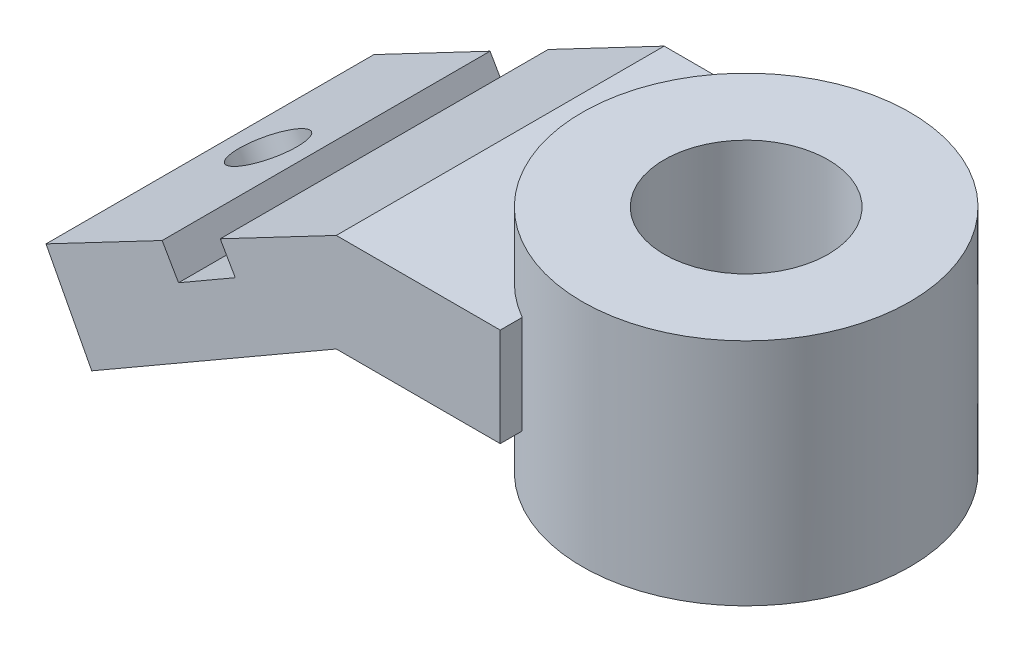
ISO-10303-21;
HEADER;
FILE_DESCRIPTION(('STEP AP214'),'2;1');
FILE_NAME('part.step','',(''),(''),'','','');
FILE_SCHEMA(('AUTOMOTIVE_DESIGN { 1 0 10303 214 1 1 1 1 }'));
ENDSEC;
DATA;
#1=APPLICATION_CONTEXT('core data for automotive mechanical design processes');
#2=APPLICATION_PROTOCOL_DEFINITION('international standard','automotive_design',2000,#1);
#3=PRODUCT_CONTEXT('',#1,'mechanical');
#4=PRODUCT('Part','Part','',(#3));
#5=PRODUCT_RELATED_PRODUCT_CATEGORY('part','',(#4));
#6=PRODUCT_DEFINITION_FORMATION('','',#4);
#7=PRODUCT_DEFINITION_CONTEXT('part definition',#1,'design');
#8=PRODUCT_DEFINITION('design','',#6,#7);
#9=PRODUCT_DEFINITION_SHAPE('','',#8);
#10=(LENGTH_UNIT() NAMED_UNIT(*) SI_UNIT(.MILLI.,.METRE.));
#11=(NAMED_UNIT(*) PLANE_ANGLE_UNIT() SI_UNIT($,.RADIAN.));
#12=(NAMED_UNIT(*) SI_UNIT($,.STERADIAN.) SOLID_ANGLE_UNIT());
#13=UNCERTAINTY_MEASURE_WITH_UNIT(LENGTH_MEASURE(1.E-05),#10,'distance_accuracy_value','');
#14=(GEOMETRIC_REPRESENTATION_CONTEXT(3) GLOBAL_UNCERTAINTY_ASSIGNED_CONTEXT((#13)) GLOBAL_UNIT_ASSIGNED_CONTEXT((#10,
#11,#12)) REPRESENTATION_CONTEXT('',''));
#15=CARTESIAN_POINT('',(0.,0.,0.));
#16=DIRECTION('',(0.,0.,1.));
#17=DIRECTION('',(1.,0.,0.));
#18=AXIS2_PLACEMENT_3D('',#15,#16,#17);
#19=CARTESIAN_POINT('',(-69.2655182091907,-8.25003005743869,25.));
#20=DIRECTION('',(0.465000601148774,-0.885310364183815,0.));
#21=DIRECTION('',(0.885310364183815,0.465000601148774,0.));
#22=AXIS2_PLACEMENT_3D('',#19,#20,#21);
#23=PLANE('',#22);
#24=DIRECTION('',(0.,0.,1.));
#25=VECTOR('',#24,1.);
#26=CARTESIAN_POINT('',(-42.7026701508798,5.70184582139558,-25.));
#27=LINE('',#26,#25);
#28=CARTESIAN_POINT('',(-42.7026701508798,5.70184582139558,-25.));
#29=VERTEX_POINT('',#28);
#30=CARTESIAN_POINT('',(-42.7026701508798,5.70184582139558,25.));
#31=VERTEX_POINT('',#30);
#32=EDGE_CURVE('E167',#29,#31,#27,.T.);
#33=ORIENTED_EDGE('',*,*,#32,.T.);
#34=DIRECTION('',(-0.885310364183815,-0.465000601148774,0.));
#35=VECTOR('',#34,1.);
#36=CARTESIAN_POINT('',(-69.2655182091907,-8.25003005743869,25.));
#37=LINE('',#36,#35);
#38=CARTESIAN_POINT('',(-25.,15.,25.));
#39=VERTEX_POINT('',#38);
#40=EDGE_CURVE('E196',#39,#31,#37,.T.);
#41=ORIENTED_EDGE('',*,*,#40,.F.);
#42=DIRECTION('',(0.,0.,-1.));
#43=VECTOR('',#42,1.);
#44=CARTESIAN_POINT('',(-25.,15.,25.));
#45=LINE('',#44,#43);
#46=CARTESIAN_POINT('',(-25.,15.,-25.));
#47=VERTEX_POINT('',#46);
#48=EDGE_CURVE('E233',#39,#47,#45,.T.);
#49=ORIENTED_EDGE('',*,*,#48,.T.);
#50=DIRECTION('',(-0.885310364183815,-0.465000601148774,0.));
#51=VECTOR('',#50,1.);
#52=CARTESIAN_POINT('',(-69.2655182091907,-8.25003005743869,-25.));
#53=LINE('',#52,#51);
#54=EDGE_CURVE('E215',#47,#29,#53,.T.);
#55=ORIENTED_EDGE('',*,*,#54,.T.);
#56=EDGE_LOOP('',(#33,#41,#49,#55));
#57=FACE_BOUND('',#56,.T.);
#58=ADVANCED_FACE('F43',(#57),#23,.F.);
#59=CARTESIAN_POINT('',(0.,0.,25.));
#60=DIRECTION('',(-1.,0.,0.));
#61=DIRECTION('',(0.,0.,1.));
#62=AXIS2_PLACEMENT_3D('',#59,#60,#61);
#63=PLANE('',#62);
#64=DIRECTION('',(0.,-1.,0.));
#65=VECTOR('',#64,1.);
#66=CARTESIAN_POINT('',(0.,25.,-21.650635094611));
#67=LINE('',#66,#65);
#68=CARTESIAN_POINT('',(0.,0.,-21.650635094611));
#69=VERTEX_POINT('',#68);
#70=CARTESIAN_POINT('',(0.,15.,-21.650635094611));
#71=VERTEX_POINT('',#70);
#72=EDGE_CURVE('E190',#69,#71,#67,.F.);
#73=ORIENTED_EDGE('',*,*,#72,.F.);
#74=DIRECTION('',(0.,0.,-1.));
#75=VECTOR('',#74,1.);
#76=CARTESIAN_POINT('',(0.,0.,25.));
#77=LINE('',#76,#75);
#78=CARTESIAN_POINT('',(0.,0.,-25.));
#79=VERTEX_POINT('',#78);
#80=EDGE_CURVE('E210',#69,#79,#77,.T.);
#81=ORIENTED_EDGE('',*,*,#80,.T.);
#82=DIRECTION('',(0.,1.,0.));
#83=VECTOR('',#82,1.);
#84=CARTESIAN_POINT('',(0.,0.,-25.));
#85=LINE('',#84,#83);
#86=CARTESIAN_POINT('',(0.,15.,-25.));
#87=VERTEX_POINT('',#86);
#88=EDGE_CURVE('E187',#79,#87,#85,.T.);
#89=ORIENTED_EDGE('',*,*,#88,.T.);
#90=DIRECTION('',(0.,0.,-1.));
#91=VECTOR('',#90,1.);
#92=CARTESIAN_POINT('',(0.,15.,25.));
#93=LINE('',#92,#91);
#94=EDGE_CURVE('E55',#71,#87,#93,.T.);
#95=ORIENTED_EDGE('',*,*,#94,.F.);
#96=EDGE_LOOP('',(#73,#81,#89,#95));
#97=FACE_BOUND('',#96,.T.);
#98=ADVANCED_FACE('F44',(#97),#63,.F.);
#99=DIRECTION('',(0.,-1.,0.));
#100=VECTOR('',#99,1.);
#101=CARTESIAN_POINT('',(0.,25.,21.650635094611));
#102=LINE('',#101,#100);
#103=CARTESIAN_POINT('',(0.,15.,21.650635094611));
#104=VERTEX_POINT('',#103);
#105=CARTESIAN_POINT('',(0.,0.,21.650635094611));
#106=VERTEX_POINT('',#105);
#107=EDGE_CURVE('E184',#104,#106,#102,.T.);
#108=ORIENTED_EDGE('',*,*,#107,.F.);
#109=CARTESIAN_POINT('',(0.,15.,25.));
#110=VERTEX_POINT('',#109);
#111=EDGE_CURVE('E11',#110,#104,#93,.T.);
#112=ORIENTED_EDGE('',*,*,#111,.F.);
#113=DIRECTION('',(0.,1.,0.));
#114=VECTOR('',#113,1.);
#115=CARTESIAN_POINT('',(0.,0.,25.));
#116=LINE('',#115,#114);
#117=CARTESIAN_POINT('',(0.,0.,25.));
#118=VERTEX_POINT('',#117);
#119=EDGE_CURVE('E192',#118,#110,#116,.T.);
#120=ORIENTED_EDGE('',*,*,#119,.F.);
#121=EDGE_CURVE('E222',#118,#106,#77,.T.);
#122=ORIENTED_EDGE('',*,*,#121,.T.);
#123=EDGE_LOOP('',(#108,#112,#120,#122));
#124=FACE_BOUND('',#123,.T.);
#125=ADVANCED_FACE('F272',(#124),#63,.F.);
#126=CARTESIAN_POINT('',(-25.,15.,25.));
#127=DIRECTION('',(0.,-1.,0.));
#128=DIRECTION('',(0.,0.,-1.));
#129=AXIS2_PLACEMENT_3D('',#126,#127,#128);
#130=PLANE('',#129);
#131=CARTESIAN_POINT('',(12.5,15.,0.));
#132=DIRECTION('',(0.,-1.,0.));
#133=DIRECTION('',(0.,0.,-1.));
#134=AXIS2_PLACEMENT_3D('',#131,#132,#133);
#135=CIRCLE('',#134,25.);
#136=EDGE_CURVE('E67',#71,#104,#135,.F.);
#137=ORIENTED_EDGE('',*,*,#136,.F.);
#138=ORIENTED_EDGE('',*,*,#94,.T.);
#139=DIRECTION('',(-1.,0.,0.));
#140=VECTOR('',#139,1.);
#141=CARTESIAN_POINT('',(-25.,15.,-25.));
#142=LINE('',#141,#140);
#143=EDGE_CURVE('E209',#87,#47,#142,.T.);
#144=ORIENTED_EDGE('',*,*,#143,.T.);
#145=ORIENTED_EDGE('',*,*,#48,.F.);
#146=DIRECTION('',(-1.,0.,0.));
#147=VECTOR('',#146,1.);
#148=CARTESIAN_POINT('',(-25.,15.,25.));
#149=LINE('',#148,#147);
#150=EDGE_CURVE('E194',#110,#39,#149,.T.);
#151=ORIENTED_EDGE('',*,*,#150,.F.);
#152=ORIENTED_EDGE('',*,*,#111,.T.);
#153=EDGE_LOOP('',(#137,#138,#144,#145,#151,#152));
#154=FACE_BOUND('',#153,.T.);
#155=ADVANCED_FACE('F238',(#154),#130,.F.);
#156=CARTESIAN_POINT('',(-60.4106474130375,-3.59909586544831,0.));
#157=DIRECTION('',(-0.465000601148774,0.885310364183815,0.));
#158=DIRECTION('',(-0.885310364183815,-0.465000601148774,0.));
#159=AXIS2_PLACEMENT_3D('',#156,#157,#158);
#160=CIRCLE('',#159,5.);
#161=CARTESIAN_POINT('',(-64.8371992339566,-5.92409887119218,0.));
#162=VERTEX_POINT('',#161);
#163=EDGE_CURVE('E158',#162,#162,#160,.T.);
#164=ORIENTED_EDGE('',*,*,#163,.F.);
#165=EDGE_LOOP('',(#164));
#166=FACE_BOUND('',#165,.T.);
#167=CARTESIAN_POINT('',(-51.5557766168843,1.05183832654207,25.));
#168=VERTEX_POINT('',#167);
#169=CARTESIAN_POINT('',(-69.2655182091907,-8.25003005743869,25.));
#170=VERTEX_POINT('',#169);
#171=EDGE_CURVE('E197',#168,#170,#37,.T.);
#172=ORIENTED_EDGE('',*,*,#171,.F.);
#173=DIRECTION('',(0.,0.,1.));
#174=VECTOR('',#173,1.);
#175=CARTESIAN_POINT('',(-51.5557766168843,1.05183832654207,-25.));
#176=LINE('',#175,#174);
#177=CARTESIAN_POINT('',(-51.5557766168843,1.05183832654207,-25.));
#178=VERTEX_POINT('',#177);
#179=EDGE_CURVE('E162',#178,#168,#176,.T.);
#180=ORIENTED_EDGE('',*,*,#179,.F.);
#181=CARTESIAN_POINT('',(-69.2655182091907,-8.25003005743869,-25.));
#182=VERTEX_POINT('',#181);
#183=EDGE_CURVE('E151',#178,#182,#53,.T.);
#184=ORIENTED_EDGE('',*,*,#183,.T.);
#185=DIRECTION('',(0.,0.,-1.));
#186=VECTOR('',#185,1.);
#187=CARTESIAN_POINT('',(-69.2655182091907,-8.25003005743869,25.));
#188=LINE('',#187,#186);
#189=EDGE_CURVE('E227',#170,#182,#188,.T.);
#190=ORIENTED_EDGE('',*,*,#189,.F.);
#191=EDGE_LOOP('',(#172,#180,#184,#190));
#192=FACE_BOUND('',#191,.T.);
#193=ADVANCED_FACE('F261',(#166,#192),#23,.F.);
#194=CARTESIAN_POINT('',(-69.2655182091907,-8.25003005743869,25.));
#195=DIRECTION('',(0.885310364183817,0.46500060114877,0.));
#196=DIRECTION('',(-0.46500060114877,0.885310364183817,0.));
#197=AXIS2_PLACEMENT_3D('',#194,#195,#196);
#198=PLANE('',#197);
#199=DIRECTION('',(0.46500060114877,-0.885310364183817,0.));
#200=VECTOR('',#199,1.);
#201=CARTESIAN_POINT('',(-69.2655182091907,-8.25003005743869,-25.));
#202=LINE('',#201,#200);
#203=CARTESIAN_POINT('',(-62.2905091919592,-21.5296855201959,-25.));
#204=VERTEX_POINT('',#203);
#205=EDGE_CURVE('E214',#182,#204,#202,.T.);
#206=ORIENTED_EDGE('',*,*,#205,.T.);
#207=DIRECTION('',(0.,0.,-1.));
#208=VECTOR('',#207,1.);
#209=CARTESIAN_POINT('',(-62.2905091919592,-21.5296855201959,25.));
#210=LINE('',#209,#208);
#211=CARTESIAN_POINT('',(-62.2905091919592,-21.5296855201959,25.));
#212=VERTEX_POINT('',#211);
#213=EDGE_CURVE('E230',#212,#204,#210,.T.);
#214=ORIENTED_EDGE('',*,*,#213,.F.);
#215=DIRECTION('',(0.46500060114877,-0.885310364183817,0.));
#216=VECTOR('',#215,1.);
#217=CARTESIAN_POINT('',(-69.2655182091907,-8.25003005743869,25.));
#218=LINE('',#217,#216);
#219=EDGE_CURVE('E203',#170,#212,#218,.T.);
#220=ORIENTED_EDGE('',*,*,#219,.F.);
#221=ORIENTED_EDGE('',*,*,#189,.T.);
#222=EDGE_LOOP('',(#206,#214,#220,#221));
#223=FACE_BOUND('',#222,.T.);
#224=ADVANCED_FACE('F260',(#223),#198,.F.);
#225=CARTESIAN_POINT('',(-25.,0.,25.));
#226=DIRECTION('',(-0.500000000000001,0.866025403784438,0.));
#227=DIRECTION('',(-0.866025403784438,-0.500000000000001,0.));
#228=AXIS2_PLACEMENT_3D('',#225,#226,#227);
#229=PLANE('',#228);
#230=CARTESIAN_POINT('',(-53.6216049479772,-16.5246913213538,0.));
#231=DIRECTION('',(-0.500000000000001,0.866025403784438,0.));
#232=DIRECTION('',(0.866025403784438,0.500000000000001,0.));
#233=AXIS2_PLACEMENT_3D('',#230,#231,#232);
#234=ELLIPSE('',#233,5.00399535907364,5.);
#235=CARTESIAN_POINT('',(-49.2880178466,-14.022693641817,0.));
#236=VERTEX_POINT('',#235);
#237=EDGE_CURVE('E50',#236,#236,#234,.T.);
#238=ORIENTED_EDGE('',*,*,#237,.T.);
#239=EDGE_LOOP('',(#238));
#240=FACE_BOUND('',#239,.T.);
#241=DIRECTION('',(0.866025403784438,0.500000000000002,0.));
#242=VECTOR('',#241,1.);
#243=CARTESIAN_POINT('',(-25.,0.,-25.));
#244=LINE('',#243,#242);
#245=CARTESIAN_POINT('',(-25.,0.,-25.));
#246=VERTEX_POINT('',#245);
#247=EDGE_CURVE('E220',#204,#246,#244,.T.);
#248=ORIENTED_EDGE('',*,*,#247,.T.);
#249=DIRECTION('',(0.,0.,-1.));
#250=VECTOR('',#249,1.);
#251=CARTESIAN_POINT('',(-25.,0.,25.));
#252=LINE('',#251,#250);
#253=CARTESIAN_POINT('',(-25.,0.,25.));
#254=VERTEX_POINT('',#253);
#255=EDGE_CURVE('E221',#254,#246,#252,.T.);
#256=ORIENTED_EDGE('',*,*,#255,.F.);
#257=DIRECTION('',(0.866025403784438,0.500000000000002,0.));
#258=VECTOR('',#257,1.);
#259=CARTESIAN_POINT('',(-25.,0.,25.));
#260=LINE('',#259,#258);
#261=EDGE_CURVE('E201',#212,#254,#260,.T.);
#262=ORIENTED_EDGE('',*,*,#261,.F.);
#263=ORIENTED_EDGE('',*,*,#213,.T.);
#264=EDGE_LOOP('',(#248,#256,#262,#263));
#265=FACE_BOUND('',#264,.T.);
#266=ADVANCED_FACE('F252',(#240,#265),#229,.F.);
#267=CARTESIAN_POINT('',(0.,0.,25.));
#268=DIRECTION('',(0.,1.,0.));
#269=DIRECTION('',(-1.,0.,0.));
#270=AXIS2_PLACEMENT_3D('',#267,#268,#269);
#271=PLANE('',#270);
#272=CARTESIAN_POINT('',(12.5,0.,0.));
#273=DIRECTION('',(0.,-1.,0.));
#274=DIRECTION('',(1.,0.,0.));
#275=AXIS2_PLACEMENT_3D('',#272,#273,#274);
#276=CIRCLE('',#275,25.);
#277=EDGE_CURVE('E171',#106,#69,#276,.T.);
#278=ORIENTED_EDGE('',*,*,#277,.F.);
#279=ORIENTED_EDGE('',*,*,#121,.F.);
#280=DIRECTION('',(1.,0.,0.));
#281=VECTOR('',#280,1.);
#282=CARTESIAN_POINT('',(0.,0.,25.));
#283=LINE('',#282,#281);
#284=EDGE_CURVE('E202',#254,#118,#283,.T.);
#285=ORIENTED_EDGE('',*,*,#284,.F.);
#286=ORIENTED_EDGE('',*,*,#255,.T.);
#287=DIRECTION('',(1.,0.,0.));
#288=VECTOR('',#287,1.);
#289=CARTESIAN_POINT('',(0.,0.,-25.));
#290=LINE('',#289,#288);
#291=EDGE_CURVE('E191',#246,#79,#290,.T.);
#292=ORIENTED_EDGE('',*,*,#291,.T.);
#293=ORIENTED_EDGE('',*,*,#80,.F.);
#294=EDGE_LOOP('',(#278,#279,#285,#286,#292,#293));
#295=FACE_BOUND('',#294,.T.);
#296=ADVANCED_FACE('F250',(#295),#271,.F.);
#297=CARTESIAN_POINT('',(0.,0.,25.));
#298=DIRECTION('',(0.,0.,-1.));
#299=DIRECTION('',(-1.,0.,0.));
#300=AXIS2_PLACEMENT_3D('',#297,#298,#299);
#301=PLANE('',#300);
#302=DIRECTION('',(0.866025403784438,0.5,0.));
#303=VECTOR('',#302,1.);
#304=CARTESIAN_POINT('',(-10.8444035099508,18.7830578570131,25.));
#305=LINE('',#304,#303);
#306=CARTESIAN_POINT('',(-49.0557766168843,-3.27828869238019,25.));
#307=VERTEX_POINT('',#306);
#308=CARTESIAN_POINT('',(-40.4024344582153,1.7177207323173,25.));
#309=VERTEX_POINT('',#308);
#310=EDGE_CURVE('E154',#307,#309,#305,.T.);
#311=ORIENTED_EDGE('',*,*,#310,.F.);
#312=DIRECTION('',(0.500000000000002,-0.866025403784438,0.));
#313=VECTOR('',#312,1.);
#314=CARTESIAN_POINT('',(-38.2113731069334,-22.0613465493933,25.));
#315=LINE('',#314,#313);
#316=EDGE_CURVE('E138',#168,#307,#315,.T.);
#317=ORIENTED_EDGE('',*,*,#316,.F.);
#318=ORIENTED_EDGE('',*,*,#171,.T.);
#319=ORIENTED_EDGE('',*,*,#219,.T.);
#320=ORIENTED_EDGE('',*,*,#261,.T.);
#321=ORIENTED_EDGE('',*,*,#284,.T.);
#322=ORIENTED_EDGE('',*,*,#119,.T.);
#323=ORIENTED_EDGE('',*,*,#150,.T.);
#324=ORIENTED_EDGE('',*,*,#40,.T.);
#325=DIRECTION('',(0.5,-0.866025403784439,0.));
#326=VECTOR('',#325,1.);
#327=CARTESIAN_POINT('',(-29.5580309482645,-17.0653371246958,25.));
#328=LINE('',#327,#326);
#329=EDGE_CURVE('E155',#31,#309,#328,.T.);
#330=ORIENTED_EDGE('',*,*,#329,.T.);
#331=EDGE_LOOP('',(#311,#317,#318,#319,#320,#321,#322,#323,#324,#330));
#332=FACE_BOUND('',#331,.T.);
#333=ADVANCED_FACE('F263',(#332),#301,.F.);
#334=CARTESIAN_POINT('',(0.,0.,-25.));
#335=DIRECTION('',(0.,0.,-1.));
#336=DIRECTION('',(-1.,0.,0.));
#337=AXIS2_PLACEMENT_3D('',#334,#335,#336);
#338=PLANE('',#337);
#339=DIRECTION('',(0.500000000000002,-0.866025403784438,0.));
#340=VECTOR('',#339,1.);
#341=CARTESIAN_POINT('',(-38.2113731069334,-22.0613465493933,-25.));
#342=LINE('',#341,#340);
#343=CARTESIAN_POINT('',(-49.0557766168843,-3.27828869238019,-25.));
#344=VERTEX_POINT('',#343);
#345=EDGE_CURVE('E132',#178,#344,#342,.T.);
#346=ORIENTED_EDGE('',*,*,#345,.T.);
#347=DIRECTION('',(0.866025403784438,0.5,0.));
#348=VECTOR('',#347,1.);
#349=CARTESIAN_POINT('',(-10.8444035099508,18.7830578570131,-25.));
#350=LINE('',#349,#348);
#351=CARTESIAN_POINT('',(-40.4024344582153,1.7177207323173,-25.));
#352=VERTEX_POINT('',#351);
#353=EDGE_CURVE('E141',#344,#352,#350,.T.);
#354=ORIENTED_EDGE('',*,*,#353,.T.);
#355=DIRECTION('',(0.5,-0.866025403784439,0.));
#356=VECTOR('',#355,1.);
#357=CARTESIAN_POINT('',(-29.5580309482645,-17.0653371246958,-25.));
#358=LINE('',#357,#356);
#359=EDGE_CURVE('E136',#29,#352,#358,.T.);
#360=ORIENTED_EDGE('',*,*,#359,.F.);
#361=ORIENTED_EDGE('',*,*,#54,.F.);
#362=ORIENTED_EDGE('',*,*,#143,.F.);
#363=ORIENTED_EDGE('',*,*,#88,.F.);
#364=ORIENTED_EDGE('',*,*,#291,.F.);
#365=ORIENTED_EDGE('',*,*,#247,.F.);
#366=ORIENTED_EDGE('',*,*,#205,.F.);
#367=ORIENTED_EDGE('',*,*,#183,.F.);
#368=EDGE_LOOP('',(#346,#354,#360,#361,#362,#363,#364,#365,#366,#367));
#369=FACE_BOUND('',#368,.T.);
#370=ADVANCED_FACE('F149',(#369),#338,.T.);
#371=CARTESIAN_POINT('',(12.5,25.,0.));
#372=DIRECTION('',(0.,-1.,0.));
#373=DIRECTION('',(0.,0.,-1.));
#374=AXIS2_PLACEMENT_3D('',#371,#372,#373);
#375=CYLINDRICAL_SURFACE('',#374,25.);
#376=CARTESIAN_POINT('',(12.5,25.,0.));
#377=DIRECTION('',(0.,1.,0.));
#378=DIRECTION('',(0.,0.,1.));
#379=AXIS2_PLACEMENT_3D('',#376,#377,#378);
#380=CIRCLE('',#379,25.);
#381=CARTESIAN_POINT('',(12.5,25.,25.));
#382=VERTEX_POINT('',#381);
#383=EDGE_CURVE('E179',#382,#382,#380,.T.);
#384=ORIENTED_EDGE('',*,*,#383,.F.);
#385=EDGE_LOOP('',(#384));
#386=FACE_BOUND('',#385,.T.);
#387=ORIENTED_EDGE('',*,*,#107,.T.);
#388=ORIENTED_EDGE('',*,*,#277,.T.);
#389=ORIENTED_EDGE('',*,*,#72,.T.);
#390=ORIENTED_EDGE('',*,*,#136,.T.);
#391=EDGE_LOOP('',(#387,#388,#389,#390));
#392=FACE_BOUND('',#391,.T.);
#393=CARTESIAN_POINT('',(12.5,-10.,0.));
#394=DIRECTION('',(0.,-1.,0.));
#395=DIRECTION('',(1.,0.,0.));
#396=AXIS2_PLACEMENT_3D('',#393,#394,#395);
#397=CIRCLE('',#396,25.);
#398=CARTESIAN_POINT('',(37.5,-9.99999999999999,0.));
#399=VERTEX_POINT('',#398);
#400=EDGE_CURVE('E177',#399,#399,#397,.T.);
#401=ORIENTED_EDGE('',*,*,#400,.F.);
#402=EDGE_LOOP('',(#401));
#403=FACE_BOUND('',#402,.T.);
#404=ADVANCED_FACE('F313',(#386,#392,#403),#375,.T.);
#405=CARTESIAN_POINT('',(0.,25.,0.));
#406=DIRECTION('',(0.,1.,0.));
#407=DIRECTION('',(0.,0.,1.));
#408=AXIS2_PLACEMENT_3D('',#405,#406,#407);
#409=PLANE('',#408);
#410=CARTESIAN_POINT('',(12.5,25.,0.));
#411=DIRECTION('',(0.,-1.,0.));
#412=DIRECTION('',(1.,0.,0.));
#413=AXIS2_PLACEMENT_3D('',#410,#411,#412);
#414=CIRCLE('',#413,12.5);
#415=CARTESIAN_POINT('',(25.,25.,0.));
#416=VERTEX_POINT('',#415);
#417=EDGE_CURVE('E168',#416,#416,#414,.T.);
#418=ORIENTED_EDGE('',*,*,#417,.T.);
#419=EDGE_LOOP('',(#418));
#420=FACE_BOUND('',#419,.T.);
#421=ORIENTED_EDGE('',*,*,#383,.T.);
#422=EDGE_LOOP('',(#421));
#423=FACE_BOUND('',#422,.T.);
#424=ADVANCED_FACE('F307',(#420,#423),#409,.T.);
#425=CARTESIAN_POINT('',(0.,-10.,0.));
#426=DIRECTION('',(0.,-1.,0.));
#427=DIRECTION('',(1.,0.,0.));
#428=AXIS2_PLACEMENT_3D('',#425,#426,#427);
#429=PLANE('',#428);
#430=CARTESIAN_POINT('',(12.5,-10.,0.));
#431=DIRECTION('',(0.,-1.,0.));
#432=DIRECTION('',(1.,0.,0.));
#433=AXIS2_PLACEMENT_3D('',#430,#431,#432);
#434=CIRCLE('',#433,12.5);
#435=CARTESIAN_POINT('',(25.,-10.,0.));
#436=VERTEX_POINT('',#435);
#437=EDGE_CURVE('E164',#436,#436,#434,.T.);
#438=ORIENTED_EDGE('',*,*,#437,.F.);
#439=EDGE_LOOP('',(#438));
#440=FACE_BOUND('',#439,.T.);
#441=ORIENTED_EDGE('',*,*,#400,.T.);
#442=EDGE_LOOP('',(#441));
#443=FACE_BOUND('',#442,.T.);
#444=ADVANCED_FACE('F303',(#440,#443),#429,.T.);
#445=CARTESIAN_POINT('',(12.5,25.,0.));
#446=DIRECTION('',(0.,-1.,0.));
#447=DIRECTION('',(1.,0.,0.));
#448=AXIS2_PLACEMENT_3D('',#445,#446,#447);
#449=CYLINDRICAL_SURFACE('',#448,12.5);
#450=ORIENTED_EDGE('',*,*,#417,.F.);
#451=EDGE_LOOP('',(#450));
#452=FACE_BOUND('',#451,.T.);
#453=ORIENTED_EDGE('',*,*,#437,.T.);
#454=EDGE_LOOP('',(#453));
#455=FACE_BOUND('',#454,.T.);
#456=ADVANCED_FACE('F302',(#452,#455),#449,.F.);
#457=CARTESIAN_POINT('',(-38.2113731069334,-22.0613465493933,-25.));
#458=DIRECTION('',(-0.866025403784437,-0.500000000000002,0.));
#459=DIRECTION('',(0.500000000000002,-0.866025403784438,0.));
#460=AXIS2_PLACEMENT_3D('',#457,#458,#459);
#461=PLANE('',#460);
#462=ORIENTED_EDGE('',*,*,#316,.T.);
#463=DIRECTION('',(0.,0.,1.));
#464=VECTOR('',#463,1.);
#465=CARTESIAN_POINT('',(-49.0557766168843,-3.27828869238019,-25.));
#466=LINE('',#465,#464);
#467=EDGE_CURVE('E135',#344,#307,#466,.T.);
#468=ORIENTED_EDGE('',*,*,#467,.F.);
#469=ORIENTED_EDGE('',*,*,#345,.F.);
#470=ORIENTED_EDGE('',*,*,#179,.T.);
#471=EDGE_LOOP('',(#462,#468,#469,#470));
#472=FACE_BOUND('',#471,.T.);
#473=ADVANCED_FACE('F131',(#472),#461,.F.);
#474=CARTESIAN_POINT('',(-29.5580309482645,-17.0653371246958,-25.));
#475=DIRECTION('',(-0.866025403784439,-0.5,0.));
#476=DIRECTION('',(0.5,-0.866025403784439,0.));
#477=AXIS2_PLACEMENT_3D('',#474,#475,#476);
#478=PLANE('',#477);
#479=ORIENTED_EDGE('',*,*,#329,.F.);
#480=ORIENTED_EDGE('',*,*,#32,.F.);
#481=ORIENTED_EDGE('',*,*,#359,.T.);
#482=DIRECTION('',(0.,0.,1.));
#483=VECTOR('',#482,1.);
#484=CARTESIAN_POINT('',(-40.4024344582153,1.7177207323173,-25.));
#485=LINE('',#484,#483);
#486=EDGE_CURVE('E56',#352,#309,#485,.T.);
#487=ORIENTED_EDGE('',*,*,#486,.T.);
#488=EDGE_LOOP('',(#479,#480,#481,#487));
#489=FACE_BOUND('',#488,.T.);
#490=ADVANCED_FACE('F264',(#489),#478,.T.);
#491=CARTESIAN_POINT('',(-10.8444035099508,18.7830578570131,-25.));
#492=DIRECTION('',(0.5,-0.866025403784438,0.));
#493=DIRECTION('',(0.866025403784438,0.5,0.));
#494=AXIS2_PLACEMENT_3D('',#491,#492,#493);
#495=PLANE('',#494);
#496=ORIENTED_EDGE('',*,*,#310,.T.);
#497=ORIENTED_EDGE('',*,*,#486,.F.);
#498=ORIENTED_EDGE('',*,*,#353,.F.);
#499=ORIENTED_EDGE('',*,*,#467,.T.);
#500=EDGE_LOOP('',(#496,#497,#498,#499));
#501=FACE_BOUND('',#500,.T.);
#502=ADVANCED_FACE('F145',(#501),#495,.F.);
#503=CARTESIAN_POINT('',(-31.8583797560222,-57.9594954332299,0.));
#504=DIRECTION('',(-0.465000601148774,0.885310364183815,0.));
#505=DIRECTION('',(-0.885310364183815,-0.465000601148774,0.));
#506=AXIS2_PLACEMENT_3D('',#503,#504,#505);
#507=CYLINDRICAL_SURFACE('',#506,5.);
#508=ORIENTED_EDGE('',*,*,#163,.T.);
#509=EDGE_LOOP('',(#508));
#510=FACE_BOUND('',#509,.T.);
#511=ORIENTED_EDGE('',*,*,#237,.F.);
#512=EDGE_LOOP('',(#511));
#513=FACE_BOUND('',#512,.T.);
#514=ADVANCED_FACE('F286',(#510,#513),#507,.F.);
#515=CLOSED_SHELL('',(#58,#98,#125,#155,#193,#224,#266,#296,#333,#370,#404,#424,#444,#456,#473,
#490,#502,#514));
#516=MANIFOLD_SOLID_BREP('B2',#515);
#517=ADVANCED_BREP_SHAPE_REPRESENTATION('',(#18,#516),#14);
#518=SHAPE_DEFINITION_REPRESENTATION(#9,#517);
ENDSEC;
END-ISO-10303-21;
